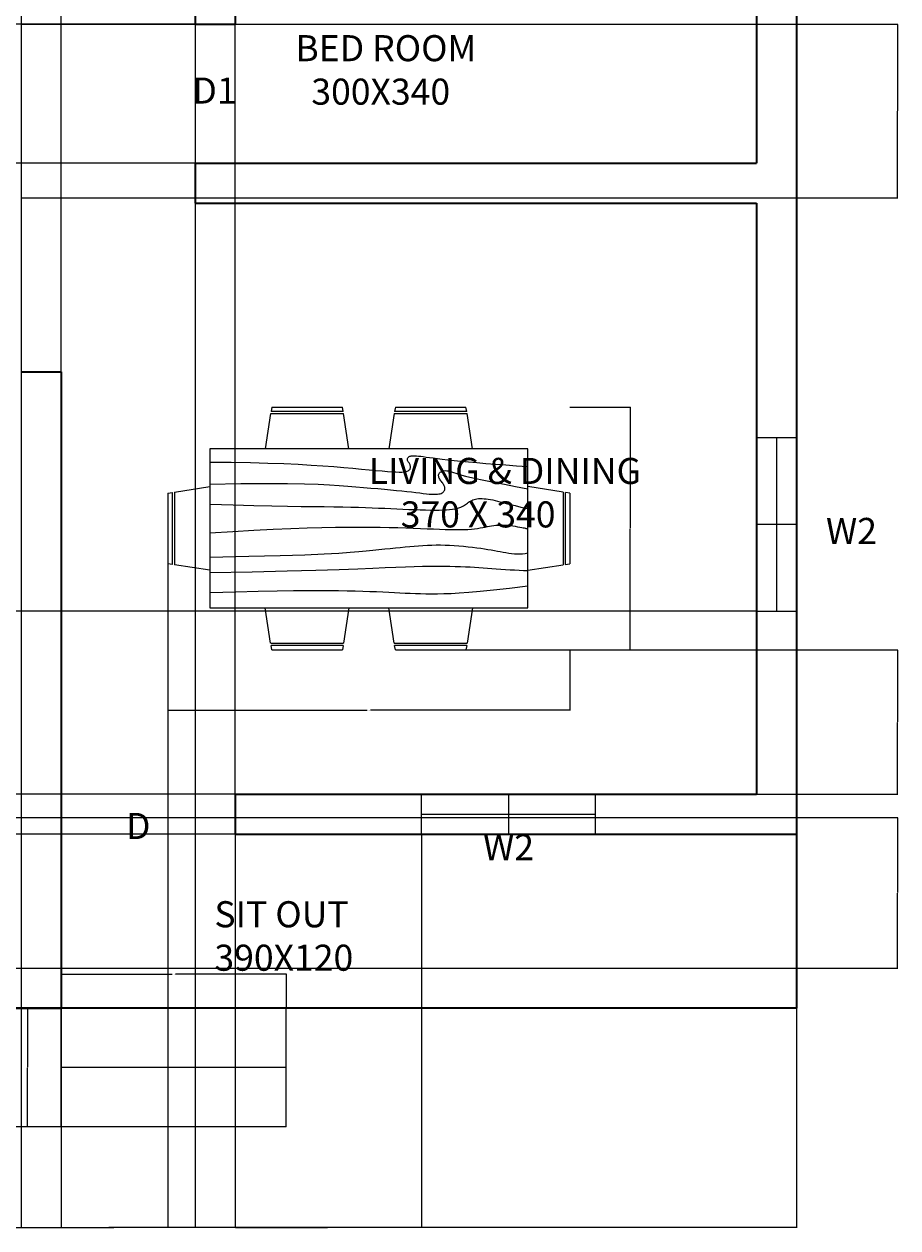
# Model space of a CAD drawing. Units: centimetres. Extents: x 575 to 1481, y 1225 to 2490.
# Tile 2 of 3: x 978 to 1481, y 1225 to 1918. Entities that reach past the tile are written whole.
import ezdxf

# ---------------------------------------------------------------- set-up
doc = ezdxf.new("R2010")
doc.units = ezdxf.units.CM
for name, color, linetype, lineweight in [('A-ANNO-DIMS', 2, 'Continuous', 18), ('A-ANNO-TEXT', 3, 'Continuous', 18), ('A-AREA-IDEN', 7, 'Continuous', 18), ('A-FLOR', 7, 'Continuous', 25), ('A-FLOR-STRS', 7, 'Continuous', 25), ('A-FURN', 8, 'Continuous', 18), ('A-GLAZ', 4, 'Continuous', 18), ('A-WALL', 7, 'Continuous', 35)]:
    doc.layers.add(name, color=color, linetype=linetype, lineweight=lineweight)
doc.styles.get("Standard").update_dxf_attribs({"font": 'arial.ttf'})
doc.dimstyles.get("Standard").update_dxf_attribs({"dimtxt": 0.18, "dimasz": 0.18, "dimexe": 0.18, "dimexo": 0.0625, "dimgap": 0.09, "dimtad": 0, "dimtih": 1, "dimtoh": 1, "dimdec": 4, "dimzin": 0, "dimdsep": 46, "dimtxsty": 'Standard', "dimcen": 0.09, "dimadec": 0, "dimazin": 0, "dimtfac": 1, "dimtdec": 4, "dimtofl": 0, "dimtmove": 0, "dimatfit": 3, "dimfxl": 1, "dimtolj": 1, "dimtzin": 0, "dimarcsym": 0})

# ---------------------------------------------------------------- blocks, each defined once
blk = doc.blocks.new('Dining Set - 36 x 72 in.')
for p, q in [((-22, 27.5), (-22.1562, 26.50042)), ((-22, 27.5), (-6, 27.5)), ((-5.8437, 26.49966), (-6, 27.5)), ((6, 27.5), (5.8438, 26.50042)), ((6, 27.5), (22, 27.5)), ((22.1563, 26.49966), (22, 27.5)), ((-22.2343, 26.00059), (-23.4847, 17.99762)), ((-22.2304, 26), (-5.7608, 26)), ((-5.8416, 26.5), (-22.1534, 26.5)), ((-4.5152, 17.99762), (-5.7655, 25.99926)), ((5.7657, 26.00059), (4.5153, 17.99762)), ((5.7696, 26), (22.2392, 26)), ((22.1584, 26.5), (5.8466, 26.5)), ((23.4848, 17.99762), (22.2345, 25.99926)), ((36, 18), (-36, 18)), ((-36, 18), (-36, -18)), ((36, -18), (36, 18)), ((-44.0006, 8.23428), (-35.9976, 9.48474)), ((-44, 8.23041), (-44, -8.23915)), ((44.0006, 8.23428), (35.9976, 9.48474)), ((44, 8.23041), (44, -8.23915)), ((-45.5, 8), (-44.5004, 8.15617)), ((-45.5, 8), (-45.5, -8)), ((-44.5, -8.15843), (-44.5, 8.15338)), ((44.5, -8.15843), (44.5, 8.15338)), ((45.5, 8), (44.5005, 8.15617)), ((45.5, 8), (45.5, -8)), ((-44.4997, -8.15631), (-45.5, -8)), ((44.4997, -8.15631), (45.5, -8)), ((-35.9976, -9.48476), (-43.9993, -8.2345)), ((35.9976, -9.48476), (43.9993, -8.2345)), ((-36, -18), (36, -18)), ((-22.2343, -26.0006), (-23.4847, -17.99762)), ((-4.5152, -17.99762), (-5.7655, -25.99928)), ((5.7657, -26.0006), (4.5153, -17.99762)), ((23.4848, -17.99762), (22.2345, -25.99928)), ((-22.2304, -26), (-5.7608, -26)), ((-22, -27.5), (-22.1562, -26.50044)), ((-5.8416, -26.5), (-22.1534, -26.5)), ((-5.8437, -26.49967), (-6, -27.5)), ((5.7696, -26), (22.2392, -26)), ((6, -27.5), (5.8438, -26.50044)), ((22.1584, -26.5), (5.8466, -26.5)), ((22.1563, -26.49967), (22, -27.5)), ((-22, -27.5), (-6, -27.5)), ((6, -27.5), (22, -27.5))]:
    blk.add_line(p, q)
for points in [[(-36, 15), (-31.1772, 14.97754), (-26.8079, 14.91406), (-22.8538, 14.81543), (-19.276, 14.6875), (-16.0362, 14.53613), (-13.0957, 14.36718), (-10.4159, 14.18652), (-7.9583, 14), (-5.6904, 13.81315), (-3.6035, 13.63021), (-1.6954, 13.45508), (0.0365, 13.29166), (1.5945, 13.14388), (2.9811, 13.01562), (4.1988, 12.9108), (5.25, 12.83333), (6.1393, 12.78613), (6.8802, 12.76823), (7.4883, 12.77767), (7.9792, 12.8125), (8.3685, 12.87077), (8.6719, 12.95052), (8.9049, 13.0498), (9.0833, 13.16666), (9.2205, 13.29899), (9.3216, 13.44401), (9.3895, 13.59879), (9.4271, 13.76041), (9.4373, 13.92594), (9.4232, 14.09245), (9.3875, 14.257), (9.3333, 14.41666), (9.2638, 14.56917), (9.1836, 14.71484), (9.0975, 14.85465), (9.0104, 14.98958), (8.9272, 15.1206), (8.8529, 15.2487), (8.7922, 15.37483), (8.75, 15.5), (8.7305, 15.62467), (8.7344, 15.74739), (8.7617, 15.86621), (8.8125, 15.97916), (8.8867, 16.08431), (8.9844, 16.17968), (9.1055, 16.26334), (9.25, 16.33333), (9.4189, 16.38802), (9.6172, 16.42708), (9.8506, 16.45052), (10.125, 16.45833), (10.4463, 16.45052), (10.8203, 16.42708), (11.2529, 16.38802), (11.75, 16.33333), (12.3184, 16.26318), (12.9694, 16.17838), (13.7151, 16.07991), (14.5677, 15.96875), (15.5395, 15.84586), (16.6426, 15.71224), (17.8893, 15.56884), (19.2917, 15.41666), (20.859, 15.25667), (22.5879, 15.08984), (24.4721, 14.91715), (26.5052, 14.73958), (28.6809, 14.5581), (30.9929, 14.3737), (33.4347, 14.18733), (36, 14)], [(-36, 10), (-28.9766, 10.14274), (-23.1725, 10.20442), (-18.4241, 10.19775), (-14.5677, 10.13541), (-11.4399, 10.03011), (-8.877, 9.89453), (-6.7154, 9.74137), (-4.7917, 9.58333), (-2.9698, 9.43082), (-1.2246, 9.28515), (0.4415, 9.14534), (2.026, 9.01041), (3.5266, 8.87939), (4.9408, 8.7513), (6.266, 8.62516), (7.5, 8.5), (8.6411, 8.37549), (9.6914, 8.2539), (10.6538, 8.13818), (11.5312, 8.03125), (12.3267, 7.93603), (13.043, 7.85547), (13.6831, 7.79248), (14.25, 7.75), (14.7471, 7.7303), (15.1797, 7.73307), (15.5537, 7.75732), (15.875, 7.80208), (16.1494, 7.86637), (16.3828, 7.94922), (16.5811, 8.04964), (16.75, 8.16666), (16.8944, 8.29915), (17.0143, 8.44531), (17.1089, 8.60319), (17.1771, 8.77083), (17.218, 8.94629), (17.2305, 9.1276), (17.2137, 9.31282), (17.1667, 9.5), (17.0895, 9.6875), (16.987, 9.875), (16.8649, 10.0625), (16.7292, 10.25), (16.5856, 10.4375), (16.4401, 10.625), (16.2985, 10.8125), (16.1667, 11), (16.05, 11.18733), (15.9518, 11.3737), (15.8752, 11.5581), (15.8229, 11.73958), (15.798, 11.91715), (15.8034, 12.08984), (15.842, 12.25667), (15.9167, 12.41666), (16.0295, 12.56836), (16.1784, 12.70833), (16.3605, 12.83268), (16.5729, 12.9375), (16.8127, 13.01888), (17.0768, 13.07291), (17.3625, 13.0957), (17.6667, 13.08333), (17.9894, 13.03312), (18.3418, 12.94726), (18.7382, 12.82918), (19.1927, 12.68229), (19.7195, 12.51001), (20.3327, 12.31575), (21.0465, 12.10294), (21.875, 11.875), (22.8357, 11.63354), (23.959, 11.37304), (25.2786, 11.08618), (26.8282, 10.76562), (28.6414, 10.40405), (30.752, 9.99414), (33.1936, 9.52856), (36, 9)], [(-36, 5.5), (-30.7157, 5.3348), (-26.069, 5.20963), (-21.9946, 5.11767), (-18.4271, 5.05208), (-15.3009, 5.00602), (-12.5508, 4.97265), (-10.1112, 4.94515), (-7.9167, 4.91666), (-5.909, 4.88167), (-4.0586, 4.83984), (-2.3429, 4.79215), (-0.7396, 4.73958), (0.7739, 4.6831), (2.22, 4.6237), (3.6213, 4.56233), (5, 4.5), (6.373, 4.43782), (7.7344, 4.3776), (9.0723, 4.32129), (10.375, 4.27083), (11.6309, 4.22819), (12.8281, 4.19531), (13.9551, 4.17415), (15, 4.16666), (15.954, 4.17448), (16.819, 4.19791), (17.6001, 4.23698), (18.3021, 4.29166), (18.9299, 4.36198), (19.4883, 4.44791), (19.9823, 4.54948), (20.4167, 4.66666), (20.7969, 4.79899), (21.1302, 4.94401), (21.4245, 5.09879), (21.6875, 5.26041), (21.9271, 5.42594), (22.1511, 5.59245), (22.3672, 5.757), (22.5834, 5.91666), (22.8065, 6.06868), (23.0404, 6.21093), (23.2879, 6.34147), (23.5521, 6.45833), (23.8358, 6.55957), (24.142, 6.64323), (24.4735, 6.70735), (24.8334, 6.75), (25.2235, 6.76969), (25.642, 6.76692), (26.0858, 6.74267), (26.5521, 6.69791), (27.0379, 6.63362), (27.5404, 6.55078), (28.0565, 6.45036), (28.5834, 6.33333), (29.1242, 6.19987), (29.7071, 6.04687), (30.3661, 5.87044), (31.1354, 5.66666), (32.0493, 5.43164), (33.142, 5.16146), (34.4475, 4.85221), (36, 4.5)], [(-36, -1), (-30.7915, -0.6591), (-26.0195, -0.38216), (-21.6519, -0.16284), (-17.6563, 0.00521), (-14.0005, 0.12833), (-10.6523, 0.21289), (-7.5796, 0.26522), (-4.75, 0.29166), (-2.134, 0.29793), (0.2878, 0.28711), (2.5317, 0.26163), (4.6146, 0.22396), (6.5529, 0.17651), (8.3633, 0.12174), (10.0623, 0.06209), (11.6667, 0), (13.1899, -0.06201), (14.6341, -0.1211), (15.9982, -0.17432), (17.2813, -0.21875), (18.4823, -0.25147), (19.6003, -0.26953), (20.6343, -0.27002), (21.5834, -0.25), (22.4481, -0.20768), (23.2357, -0.14584), (23.9549, -0.06836), (24.6146, 0.02083), (25.2235, 0.11784), (25.7904, 0.21875), (26.3241, 0.31966), (26.8334, 0.41666), (27.3265, 0.50618), (27.8099, 0.58593), (28.2894, 0.65397), (28.7709, 0.70833), (29.2601, 0.74707), (29.763, 0.76823), (30.2855, 0.76985), (30.8334, 0.75), (31.4088, 0.70784), (31.9994, 0.64713), (32.589, 0.57275), (33.1615, 0.48958), (33.7008, 0.4025), (34.1908, 0.3164), (34.6153, 0.23616), (34.9584, 0.16666), (35.2099, 0.11165), (35.3848, 0.07031), (35.504, 0.04069), (35.5886, 0.02083), (35.6594, 0.00879), (35.7377, 0.0026), (35.8442, 0.00032), (36, 0)], [(-36, -6.5), (-27.1843, -6.31267), (-20.084, -6.1263), (-14.469, -5.9419), (-10.1094, -5.76042), (-6.7752, -5.58285), (-4.2363, -5.41016), (-2.2629, -5.24333), (-0.625, -5.08334), (0.8708, -4.93099), (2.2715, -4.78646), (3.5872, -4.64974), (4.8281, -4.52084), (6.0046, -4.39974), (7.127, -4.28646), (8.2053, -4.18099), (9.25, -4.08334), (10.2705, -3.99382), (11.2734, -3.91407), (12.2647, -3.84603), (13.25, -3.79167), (14.2354, -3.75293), (15.2266, -3.73177), (16.2295, -3.73015), (17.25, -3.75), (18.2912, -3.79248), (19.3451, -3.85547), (20.4009, -3.93604), (21.4479, -4.03125), (22.4754, -4.13819), (23.4727, -4.25391), (24.4289, -4.37549), (25.3334, -4.5), (26.1785, -4.62492), (26.9694, -4.74935), (27.7145, -4.87281), (28.4219, -4.99479), (29.1, -5.11483), (29.7572, -5.23242), (30.4016, -5.34709), (31.0417, -5.45834), (31.6837, -5.56437), (32.3262, -5.65821), (32.9658, -5.73153), (33.599, -5.77604), (34.2224, -5.78345), (34.8327, -5.74545), (35.4264, -5.65373), (36, -5.5)], [(-36, -10), (-26.4022, -9.81299), (-18.4675, -9.62891), (-11.9839, -9.45069), (-6.7396, -9.28125), (-2.5226, -9.12354), (0.8789, -8.98047), (3.6769, -8.85498), (6.0833, -8.75), (8.2767, -8.66765), (10.3021, -8.60677), (12.1712, -8.56543), (13.8958, -8.54167), (15.4876, -8.53353), (16.9583, -8.53907), (18.3197, -8.55632), (19.5834, -8.58334), (20.7616, -8.61841), (21.8685, -8.66081), (22.9188, -8.71004), (23.9271, -8.76563), (24.9081, -8.82707), (25.8763, -8.89388), (26.8465, -8.96558), (27.8334, -9.04167), (28.8474, -9.12118), (29.8828, -9.20117), (30.93, -9.27824), (31.9792, -9.34896), (33.0205, -9.40991), (34.0443, -9.45768), (35.0407, -9.48885), (36, -9.5)], [(-36, -14.5), (-30.0881, -14.33513), (-25.0332, -14.21224), (-20.7312, -14.12647), (-17.0781, -14.07292), (-13.97, -14.04671), (-11.3027, -14.04297), (-8.9724, -14.05681), (-6.875, -14.08334), (-4.9224, -14.11833), (-3.0905, -14.16016), (-1.3709, -14.20785), (0.2448, -14.26042), (1.7647, -14.3169), (3.1973, -14.3763), (4.5507, -14.43767), (5.8333, -14.5), (7.0554, -14.5621), (8.235, -14.62175), (9.3922, -14.67652), (10.5469, -14.72396), (11.7192, -14.76164), (12.929, -14.78711), (14.1965, -14.79794), (15.5417, -14.79167), (16.9933, -14.76424), (18.6152, -14.70508), (20.4804, -14.60197), (22.6615, -14.44271), (25.2312, -14.21509), (28.2624, -13.9069), (31.8277, -13.50594), (36, -13)]]:
    blk.add_lwpolyline(points)
blk = doc.blocks.new('WIN-W2-100CM')
for p, q in [((0, 0), (0, 23)), ((50, 23), (50, 0)), ((100, 0), (100, 23)), ((0, 11.5), (100, 11.5))]:
    blk.add_line(p, q)
blk = doc.blocks.new('ENTRY-STEPS')
for p, q in [((0, 0), (0, 68.38)), ((129.45, 68.38), (0, 68.38)), ((129.45, 0), (129.45, 68.38)), ((129.45, 34.19), (0, 34.19)), ((129.45, 0), (0, 0))]:
    blk.add_line(p, q)
blk = doc.blocks.new('*D16')
at = {"layer": 'A-ANNO-DIMS', "color": 0, "lineweight": -2, "transparency": 16777216}
for p, q in [((999.46, 1351.63), (999.46, 1371.16)), ((999.64, 1370.98), (1063.14, 1370.98)), ((1128.73, 1370.98), (1065.23, 1370.98)), ((1128.91, 1351.63), (1128.91, 1371.16))]:
    blk.add_line(p, q, dxfattribs=at)
at = {"layer": 'A-ANNO-DIMS', "color": 0, "transparency": 16777216}
for points in [[(999.64, 1371.01), (999.64, 1370.95), (999.46, 1370.98)], [(1128.73, 1371.01), (1128.73, 1370.95), (1128.91, 1370.98)]]:
    blk.add_solid(points, dxfattribs=at)
at = {"layer": 'Defpoints', "color": 0, "transparency": 16777216}
for p in [(1128.91, 1370.98), (999.46, 1351.57), (1128.91, 1351.57)]:
    blk.add_point(p, dxfattribs=at)
at = {"layer": 'A-ANNO-DIMS', "color": 0, "transparency": 16777216, "insert": (1064.18, 1370.98), "char_height": 0.18, "attachment_point": 5}
blk.add_mtext('\\A1;STEPS 129 TYP.', dxfattribs=at)
blk = doc.blocks.new('*D17')
at = {"layer": 'A-ANNO-DIMS', "color": 0, "lineweight": -2, "transparency": 16777216}
for p, q in [((999.39, 1351.57), (979.86, 1351.57)), ((980.04, 1351.39), (980.04, 1317.56)), ((980.04, 1283.37), (980.04, 1317.19)), ((999.39, 1283.19), (979.86, 1283.19))]:
    blk.add_line(p, q, dxfattribs=at)
at = {"layer": 'A-ANNO-DIMS', "color": 0, "transparency": 16777216}
for points in [[(980.01, 1351.39), (980.07, 1351.39), (980.04, 1351.57)], [(980.01, 1283.37), (980.07, 1283.37), (980.04, 1283.19)]]:
    blk.add_solid(points, dxfattribs=at)
at = {"layer": 'Defpoints', "color": 0, "transparency": 16777216}
for p in [(980.04, 1351.57), (999.46, 1351.57), (999.46, 1283.19)]:
    blk.add_point(p, dxfattribs=at)
at = {"layer": 'A-ANNO-DIMS', "color": 0, "transparency": 16777216, "insert": (980.04, 1317.38), "char_height": 0.18, "attachment_point": 5}
blk.add_mtext('\\A1;68 TYP.', dxfattribs=at)
blk = doc.blocks.new('*D22')
at = {"layer": 'A-ANNO-DIMS', "color": 0, "lineweight": -2, "transparency": 16777216}
for p, q in [((1060.8, 1557.52), (1060.8, 1522.73)), ((1291.94, 1557.52), (1291.94, 1522.73)), ((1060.98, 1522.91), (1175.35, 1522.91)), ((1291.76, 1522.91), (1177.39, 1522.91))]:
    blk.add_line(p, q, dxfattribs=at)
at = {"layer": 'A-ANNO-DIMS', "color": 0, "transparency": 16777216}
for points in [[(1060.98, 1522.94), (1060.98, 1522.88), (1060.8, 1522.91)], [(1291.76, 1522.94), (1291.76, 1522.88), (1291.94, 1522.91)]]:
    blk.add_solid(points, dxfattribs=at)
at = {"layer": 'Defpoints', "color": 0, "transparency": 16777216}
for p in [(1060.8, 1557.58), (1291.94, 1557.58), (1291.94, 1522.91)]:
    blk.add_point(p, dxfattribs=at)
at = {"layer": 'A-ANNO-DIMS', "color": 0, "transparency": 16777216, "insert": (1176.37, 1522.91), "char_height": 0.18, "attachment_point": 5}
blk.add_mtext('\\A1;DINING SET 231', dxfattribs=at)
blk = doc.blocks.new('*D23')
at = {"layer": 'A-ANNO-DIMS', "color": 0, "lineweight": -2, "transparency": 16777216}
for p, q in [((1292, 1697.28), (1326.79, 1697.28)), ((1326.61, 1697.1), (1326.61, 1627.61)), ((1326.61, 1557.76), (1326.61, 1627.25)), ((1292, 1557.58), (1326.79, 1557.58))]:
    blk.add_line(p, q, dxfattribs=at)
at = {"layer": 'A-ANNO-DIMS', "color": 0, "transparency": 16777216}
for points in [[(1326.58, 1697.1), (1326.64, 1697.1), (1326.61, 1697.28)], [(1326.58, 1557.76), (1326.64, 1557.76), (1326.61, 1557.58)]]:
    blk.add_solid(points, dxfattribs=at)
at = {"layer": 'Defpoints', "color": 0, "transparency": 16777216}
for p in [(1291.94, 1697.28), (1326.61, 1697.28), (1291.94, 1557.58)]:
    blk.add_point(p, dxfattribs=at)
at = {"layer": 'A-ANNO-DIMS', "color": 0, "transparency": 16777216, "insert": (1326.61, 1627.43), "char_height": 0.18, "attachment_point": 5}
blk.add_mtext('\\A1;140', dxfattribs=at)
blk = doc.blocks.new('*D28')
at = {"layer": 'A-ANNO-DIMS', "color": 0, "lineweight": -2, "transparency": 16777216}
for p, q in [((633.46, 1351.5), (633.46, 1225.06)), ((1422.46, 1351.5), (1422.46, 1225.06)), ((633.64, 1225.24), (1027.67, 1225.24)), ((1422.28, 1225.24), (1028.25, 1225.24))]:
    blk.add_line(p, q, dxfattribs=at)
at = {"layer": 'A-ANNO-DIMS', "color": 0, "transparency": 16777216}
for points in [[(633.64, 1225.27), (633.64, 1225.21), (633.46, 1225.24)], [(1422.28, 1225.27), (1422.28, 1225.21), (1422.46, 1225.24)]]:
    blk.add_solid(points, dxfattribs=at)
at = {"layer": 'Defpoints', "color": 0, "transparency": 16777216}
for p in [(633.46, 1351.57), (1422.46, 1351.57), (1422.46, 1225.24)]:
    blk.add_point(p, dxfattribs=at)
at = {"layer": 'A-ANNO-DIMS', "color": 0, "transparency": 16777216, "insert": (1027.96, 1225.24), "char_height": 0.18, "attachment_point": 5}
blk.add_mtext('\\A1;789', dxfattribs=at)
blk = doc.blocks.new('*D29')
at = {"layer": 'A-ANNO-DIMS', "color": 0, "lineweight": -2, "transparency": 16777216}
for p, q in [((959.64, 2431.95), (575.33, 2431.95)), ((575.51, 2431.77), (575.51, 1857.75)), ((575.51, 1283.37), (575.51, 1857.38)), ((999.39, 1283.19), (575.33, 1283.19))]:
    blk.add_line(p, q, dxfattribs=at)
at = {"layer": 'A-ANNO-DIMS', "color": 0, "transparency": 16777216}
for points in [[(575.48, 2431.77), (575.54, 2431.77), (575.51, 2431.95)], [(575.48, 1283.37), (575.54, 1283.37), (575.51, 1283.19)]]:
    blk.add_solid(points, dxfattribs=at)
at = {"layer": 'Defpoints', "color": 0, "transparency": 16777216}
for p in [(575.51, 2431.95), (959.71, 2431.95), (999.46, 1283.19)]:
    blk.add_point(p, dxfattribs=at)
at = {"layer": 'A-ANNO-DIMS', "color": 0, "transparency": 16777216, "insert": (575.51, 1857.57), "char_height": 0.18, "attachment_point": 5}
blk.add_mtext('\\A1;1148.8', dxfattribs=at)
blk = doc.blocks.new('*D31')
at = {"layer": 'A-ANNO-DIMS', "color": 0, "lineweight": -2, "transparency": 16777216}
for p, q in [((1099.46, 1451.5), (1099.46, 1225.06)), ((1206.74, 1451.5), (1206.74, 1225.06)), ((1099.64, 1225.24), (1152.64, 1225.24)), ((1206.56, 1225.24), (1153.55, 1225.24))]:
    blk.add_line(p, q, dxfattribs=at)
at = {"layer": 'A-ANNO-DIMS', "color": 0, "transparency": 16777216}
for points in [[(1099.64, 1225.27), (1099.64, 1225.21), (1099.46, 1225.24)], [(1206.56, 1225.27), (1206.56, 1225.21), (1206.74, 1225.24)]]:
    blk.add_solid(points, dxfattribs=at)
at = {"layer": 'Defpoints', "color": 0, "transparency": 16777216}
for p in [(1099.46, 1451.57), (1206.74, 1451.57), (1206.74, 1225.24)]:
    blk.add_point(p, dxfattribs=at)
at = {"layer": 'A-ANNO-DIMS', "color": 0, "transparency": 16777216, "insert": (1153.1, 1225.24), "char_height": 0.18, "attachment_point": 5}
blk.add_mtext('\\A1;107.28', dxfattribs=at)
blk = doc.blocks.new('*D32')
at = {"layer": 'A-ANNO-DIMS', "color": 0, "lineweight": -2, "transparency": 16777216}
for p, q in [((656.52, 1461.2), (1480.59, 1461.2)), ((1480.41, 1461.02), (1480.41, 1418.07)), ((1480.41, 1374.75), (1480.41, 1417.7)), ((656.52, 1374.57), (1480.59, 1374.57))]:
    blk.add_line(p, q, dxfattribs=at)
at = {"layer": 'A-ANNO-DIMS', "color": 0, "transparency": 16777216}
for points in [[(1480.38, 1461.02), (1480.44, 1461.02), (1480.41, 1461.2)], [(1480.38, 1374.75), (1480.44, 1374.75), (1480.41, 1374.57)]]:
    blk.add_solid(points, dxfattribs=at)
at = {"layer": 'Defpoints', "color": 0, "transparency": 16777216}
for p in [(656.46, 1461.2), (1480.41, 1461.2), (656.46, 1374.57)]:
    blk.add_point(p, dxfattribs=at)
at = {"layer": 'A-ANNO-DIMS', "color": 0, "transparency": 16777216, "insert": (1480.41, 1417.88), "char_height": 0.18, "attachment_point": 5}
blk.add_mtext('\\A1;86.63', dxfattribs=at)
blk = doc.blocks.new('*D37')
at = {"layer": 'A-ANNO-DIMS', "color": 0, "lineweight": -2, "transparency": 16777216}
for p, q in [((1076.46, 2363.5), (1076.46, 1225.06)), ((976.46, 2340.5), (976.46, 1225.06)), ((976.64, 1225.24), (1026.18, 1225.24)), ((1076.28, 1225.24), (1026.74, 1225.24))]:
    blk.add_line(p, q, dxfattribs=at)
at = {"layer": 'A-ANNO-DIMS', "color": 0, "transparency": 16777216}
for points in [[(976.64, 1225.27), (976.64, 1225.21), (976.46, 1225.24)], [(1076.28, 1225.27), (1076.28, 1225.21), (1076.46, 1225.24)]]:
    blk.add_solid(points, dxfattribs=at)
at = {"layer": 'Defpoints', "color": 0, "transparency": 16777216}
for p in [(1076.46, 2363.57), (976.46, 2340.57), (1076.46, 1225.24)]:
    blk.add_point(p, dxfattribs=at)
at = {"layer": 'A-ANNO-DIMS', "color": 0, "transparency": 16777216, "insert": (1026.46, 1225.24), "char_height": 0.18, "attachment_point": 5}
blk.add_mtext('\\A1;100', dxfattribs=at)
blk = doc.blocks.new('*D39')
at = {"layer": 'A-ANNO-DIMS', "color": 0, "lineweight": -2, "transparency": 16777216}
for p, q in [((1399.39, 1579.79), (575.33, 1579.79)), ((575.51, 1579.61), (575.51, 1527.36)), ((575.51, 1474.75), (575.51, 1527)), ((1399.39, 1474.57), (575.33, 1474.57))]:
    blk.add_line(p, q, dxfattribs=at)
at = {"layer": 'A-ANNO-DIMS', "color": 0, "transparency": 16777216}
for points in [[(575.48, 1579.61), (575.54, 1579.61), (575.51, 1579.79)], [(575.48, 1474.75), (575.54, 1474.75), (575.51, 1474.57)]]:
    blk.add_solid(points, dxfattribs=at)
at = {"layer": 'Defpoints', "color": 0, "transparency": 16777216}
for p in [(575.51, 1579.79), (1399.46, 1579.79), (1399.46, 1474.57)]:
    blk.add_point(p, dxfattribs=at)
at = {"layer": 'A-ANNO-DIMS', "color": 0, "transparency": 16777216, "insert": (575.51, 1527.18), "char_height": 0.18, "attachment_point": 5}
blk.add_mtext('\\A1;105.22', dxfattribs=at)
blk = doc.blocks.new('*D40')
at = {"layer": 'A-ANNO-DIMS', "color": 0, "lineweight": -2, "transparency": 16777216}
for p, q in [((1399.39, 1925.38), (575.33, 1925.38)), ((575.51, 1925.2), (575.51, 1881.66)), ((575.51, 1837.75), (575.51, 1881.29)), ((1399.39, 1837.57), (575.33, 1837.57))]:
    blk.add_line(p, q, dxfattribs=at)
at = {"layer": 'A-ANNO-DIMS', "color": 0, "transparency": 16777216}
for points in [[(575.48, 1925.2), (575.54, 1925.2), (575.51, 1925.38)], [(575.48, 1837.75), (575.54, 1837.75), (575.51, 1837.57)]]:
    blk.add_solid(points, dxfattribs=at)
at = {"layer": 'Defpoints', "color": 0, "transparency": 16777216}
for p in [(575.51, 1925.38), (1399.46, 1925.38), (1399.46, 1837.57)]:
    blk.add_point(p, dxfattribs=at)
at = {"layer": 'A-ANNO-DIMS', "color": 0, "transparency": 16777216, "insert": (575.51, 1881.47), "char_height": 0.18, "attachment_point": 5}
blk.add_mtext('\\A1;87.82', dxfattribs=at)
blk = doc.blocks.new('*D42')
at = {"layer": 'A-ANNO-DIMS', "color": 0, "lineweight": -2, "transparency": 16777216}
for p, q in [((976.52, 1917.57), (1480.59, 1917.57)), ((1480.41, 1917.39), (1480.41, 1867.75)), ((1480.41, 1817.75), (1480.41, 1867.38)), ((976.52, 1817.57), (1480.59, 1817.57))]:
    blk.add_line(p, q, dxfattribs=at)
at = {"layer": 'A-ANNO-DIMS', "color": 0, "transparency": 16777216}
for points in [[(1480.38, 1917.39), (1480.44, 1917.39), (1480.41, 1917.57)], [(1480.38, 1817.75), (1480.44, 1817.75), (1480.41, 1817.57)]]:
    blk.add_solid(points, dxfattribs=at)
at = {"layer": 'Defpoints', "color": 0, "transparency": 16777216}
for p in [(976.46, 1917.57), (1480.41, 1917.57), (976.46, 1817.57)]:
    blk.add_point(p, dxfattribs=at)
at = {"layer": 'A-ANNO-DIMS', "color": 0, "transparency": 16777216, "insert": (1480.41, 1867.57), "char_height": 0.18, "attachment_point": 5}
blk.add_mtext('\\A1;100', dxfattribs=at)
blk = doc.blocks.new('*D46')
at = {"layer": 'A-ANNO-DIMS', "color": 0, "lineweight": -2, "transparency": 16777216}
for p, q in [((1076.39, 1917.57), (575.33, 1917.57)), ((575.51, 1917.39), (575.51, 1877.75)), ((575.51, 1837.75), (575.51, 1877.38)), ((1076.39, 1837.57), (575.33, 1837.57))]:
    blk.add_line(p, q, dxfattribs=at)
at = {"layer": 'A-ANNO-DIMS', "color": 0, "transparency": 16777216}
for points in [[(575.48, 1917.39), (575.54, 1917.39), (575.51, 1917.57)], [(575.48, 1837.75), (575.54, 1837.75), (575.51, 1837.57)]]:
    blk.add_solid(points, dxfattribs=at)
at = {"layer": 'Defpoints', "color": 0, "transparency": 16777216}
for p in [(575.51, 1917.57), (1076.46, 1917.57), (1076.46, 1837.57)]:
    blk.add_point(p, dxfattribs=at)
at = {"layer": 'A-ANNO-DIMS', "color": 0, "transparency": 16777216, "insert": (575.51, 1877.57), "char_height": 0.18, "attachment_point": 5}
blk.add_mtext('\\A1;80', dxfattribs=at)
blk = doc.blocks.new('*D48')
at = {"layer": 'A-ANNO-DIMS', "color": 0, "lineweight": -2, "transparency": 16777216}
for p, q in [((999.46, 1351.63), (999.46, 2490.08)), ((999.64, 2489.9), (1049.18, 2489.9)), ((1099.28, 2489.9), (1049.74, 2489.9)), ((1099.46, 1451.63), (1099.46, 2490.08))]:
    blk.add_line(p, q, dxfattribs=at)
at = {"layer": 'A-ANNO-DIMS', "color": 0, "transparency": 16777216}
for points in [[(999.64, 2489.93), (999.64, 2489.87), (999.46, 2489.9)], [(1099.28, 2489.93), (1099.28, 2489.87), (1099.46, 2489.9)]]:
    blk.add_solid(points, dxfattribs=at)
at = {"layer": 'Defpoints', "color": 0, "transparency": 16777216}
for p in [(1099.46, 2489.9), (1099.46, 1451.57), (999.46, 1351.57)]:
    blk.add_point(p, dxfattribs=at)
at = {"layer": 'A-ANNO-DIMS', "color": 0, "transparency": 16777216, "insert": (1049.46, 2489.9), "char_height": 0.18, "attachment_point": 5}
blk.add_mtext('\\A1;100', dxfattribs=at)
blk = doc.blocks.new('*D55')
at = {"layer": 'A-ANNO-DIMS', "color": 0, "lineweight": -2, "transparency": 16777216}
for p, q in [((999.46, 1717.5), (999.46, 1225.06)), ((1060.8, 1607.05), (1060.8, 1225.06)), ((999.64, 1225.24), (1029.73, 1225.24)), ((1060.62, 1225.24), (1030.52, 1225.24))]:
    blk.add_line(p, q, dxfattribs=at)
at = {"layer": 'A-ANNO-DIMS', "color": 0, "transparency": 16777216}
for points in [[(999.64, 1225.27), (999.64, 1225.21), (999.46, 1225.24)], [(1060.62, 1225.27), (1060.62, 1225.21), (1060.8, 1225.24)]]:
    blk.add_solid(points, dxfattribs=at)
at = {"layer": 'Defpoints', "color": 0, "transparency": 16777216}
for p in [(999.46, 1717.57), (1060.8, 1607.11), (1060.8, 1225.24)]:
    blk.add_point(p, dxfattribs=at)
at = {"layer": 'A-ANNO-DIMS', "color": 0, "transparency": 16777216, "insert": (1030.13, 1225.24), "char_height": 0.18, "attachment_point": 5}
blk.add_mtext('\\A1;61.34', dxfattribs=at)
blk = doc.blocks.new('*D56')
at = {"layer": 'A-ANNO-DIMS', "color": 0, "lineweight": -2, "transparency": 16777216}
for p, q in [((1232.31, 1557.58), (1480.59, 1557.58)), ((1480.41, 1557.4), (1480.41, 1516.25)), ((1480.41, 1474.75), (1480.41, 1515.89)), ((1399.52, 1474.57), (1480.59, 1474.57))]:
    blk.add_line(p, q, dxfattribs=at)
at = {"layer": 'A-ANNO-DIMS', "color": 0, "transparency": 16777216}
for points in [[(1480.38, 1557.4), (1480.44, 1557.4), (1480.41, 1557.58)], [(1480.38, 1474.75), (1480.44, 1474.75), (1480.41, 1474.57)]]:
    blk.add_solid(points, dxfattribs=at)
at = {"layer": 'Defpoints', "color": 0, "transparency": 16777216}
for p in [(1232.25, 1557.58), (1480.41, 1557.58), (1399.46, 1474.57)]:
    blk.add_point(p, dxfattribs=at)
at = {"layer": 'A-ANNO-DIMS', "color": 0, "transparency": 16777216, "insert": (1480.41, 1516.07), "char_height": 0.18, "attachment_point": 5}
blk.add_mtext('\\A1;83.01', dxfattribs=at)
blk = doc.blocks.new('*D57')
at = {"layer": 'A-ANNO-DIMS', "color": 0, "lineweight": -2, "transparency": 16777216}
for p, q in [((1422.39, 1451.57), (575.33, 1451.57)), ((575.51, 1451.39), (575.51, 1401.75)), ((575.51, 1351.75), (575.51, 1401.38)), ((1422.39, 1351.57), (575.33, 1351.57))]:
    blk.add_line(p, q, dxfattribs=at)
at = {"layer": 'A-ANNO-DIMS', "color": 0, "transparency": 16777216}
for points in [[(575.48, 1451.39), (575.54, 1451.39), (575.51, 1451.57)], [(575.48, 1351.75), (575.54, 1351.75), (575.51, 1351.57)]]:
    blk.add_solid(points, dxfattribs=at)
at = {"layer": 'Defpoints', "color": 0, "transparency": 16777216}
for p in [(575.51, 1451.57), (1422.46, 1451.57), (1422.46, 1351.57)]:
    blk.add_point(p, dxfattribs=at)
at = {"layer": 'A-ANNO-DIMS', "color": 0, "transparency": 16777216, "insert": (575.51, 1401.57), "char_height": 0.18, "attachment_point": 5}
blk.add_mtext('\\A1;100', dxfattribs=at)

msp = doc.modelspace()

# ---------------------------------------------------------------- linework, layer by layer
at = {"layer": 'A-FLOR'}
msp.add_line((999.457, 1351.566), (1422.457, 1351.566), dxfattribs=at)
at = {"layer": 'A-GLAZ'}
for p, q in [((1399.457, 1679.7906), (1399.457, 1579.7906)), ((1422.457, 1579.7906), (1422.457, 1679.7906))]:
    msp.add_line(p, q, dxfattribs=at)
at = {"layer": 'A-WALL'}
for p, q in [((1076.457, 2363.566), (1076.457, 1917.566)), ((1422.457, 2363.566), (1422.457, 1351.566)), ((1399.457, 2340.566), (1399.457, 1837.566)), ((1099.457, 2177.566), (1099.457, 1917.566)), ((1076.457, 1917.566), (1099.457, 1917.566)), ((1076.457, 1837.566), (1399.457, 1837.566)), ((1076.457, 1837.566), (1076.457, 1814.566)), ((1076.457, 1814.566), (1399.457, 1814.566)), ((1399.457, 1814.566), (1399.457, 1474.566)), ((976.457, 1717.566), (999.457, 1717.566)), ((999.457, 1717.566), (999.457, 1351.566)), ((1099.457, 1474.566), (1399.457, 1474.566)), ((1099.457, 1474.566), (1099.457, 1451.566)), ((1099.457, 1451.566), (1422.457, 1451.566)), ((633.457, 1351.566), (999.457, 1351.566))]:
    msp.add_line(p, q, dxfattribs=at)

# ---------------------------------------------------------------- block references
at = {"layer": 'A-FLOR-STRS'}
msp.add_blockref('ENTRY-STEPS', (999.4565, 1283.1864), dxfattribs=at)
at = {"layer": 'A-FURN', "xscale": 2.54, "yscale": 2.54, "zscale": 2.54}
msp.add_blockref('Dining Set - 36 x 72 in.', (1176.3676, 1627.4299), dxfattribs=at)
at = {"layer": 'A-GLAZ', "rotation": 269.9999999999999}
msp.add_blockref('WIN-W2-100CM', (1399.4569, 1679.7901), dxfattribs=at)
at = {"layer": 'A-GLAZ'}
msp.add_blockref('WIN-W2-100CM', (1206.739, 1451.566), dxfattribs=at)

# ---------------------------------------------------------------- texts
at = {"layer": 'A-ANNO-TEXT', "char_height": 15, "attachment_point": 1}
for s, insert in [('D1', (1074.889, 1886.824)), ('W2', (1439.3315, 1633.4884)), ('D', (1036.6686, 1463.7707)), ('W2', (1242.0708, 1451.566))]:
    msp.add_mtext_dynamic_manual_height_columns(s, width=230.89075, gutter_width=12.5, heights=[0], dxfattribs=dict(at, insert=insert))
at = {"layer": 'A-AREA-IDEN', "char_height": 15, "attachment_point": 1}
for s, heights, insert in [('BED ROOM\\P  300X340', [68.7606], (1134.1082, 1911.2008)), ('LIVING & DINING\\P    370 X 340', [0], (1176.3676, 1668.0132)), ('SIT OUT \\P390X120', [0], (1087.5366, 1412.9951))]:
    msp.add_mtext_dynamic_manual_height_columns(s, width=230.89075, gutter_width=12.5, heights=heights, dxfattribs=dict(at, insert=insert))

# ---------------------------------------------------------------- dimensions: what is measured, and where the dimension line sits
at = {"layer": 'A-ANNO-DIMS'}
for base, p1, p2, override, picture, middle in [((1099.457, 2489.8956), (999.457, 1351.566), (1099.457, 1451.566), {"dimdec": 0, "dimlfac": 1, "dimrnd": 0, "dimzin": 0, "dimdsep": 46, "dimlunit": 2}, '*D48', (1049.457, 2489.8956)), ((1076.457, 1225.2364), (976.457, 2340.566), (1076.457, 2363.566), {"dimdec": 0, "dimlfac": 1, "dimrnd": 0, "dimzin": 0, "dimdsep": 46, "dimlunit": 2}, '*D37', (1026.457, 1225.2364)), ((1060.7976, 1225.2364), (999.457, 1717.566), (1060.7976, 1607.1099), {"dimdec": 2, "dimlfac": 1, "dimrnd": 0, "dimzin": 0, "dimdsep": 46, "dimlunit": 2}, '*D55', (1030.1273, 1225.2364)), ((1206.7385, 1225.2364), (1099.457, 1451.566), (1206.7385, 1451.566), {"dimdec": 2, "dimlfac": 1, "dimrnd": 0, "dimzin": 0, "dimdsep": 46, "dimlunit": 2}, '*D31', (1153.0978, 1225.2364)), ((1422.457, 1225.2364), (633.457, 1351.566), (1422.457, 1351.566), {"dimdec": 0, "dimlfac": 1, "dimrnd": 0, "dimzin": 0, "dimdsep": 46, "dimlunit": 2}, '*D28', (1027.957, 1225.2364))]:
    dim = msp.add_linear_dim(base=base, p1=p1, p2=p2, dimstyle='Standard', override=override, dxfattribs=at)
    dim.commit()
    dim.dimension.update_dxf_attribs({"geometry": picture, "text_midpoint": middle})
for base, p1, p2, override, picture, middle in [((575.507, 2431.9456), (999.457, 1283.1864), (959.7054, 2431.9456), {"dimdec": 1, "dimlfac": 1, "dimrnd": 0, "dimzin": 0, "dimdsep": 46, "dimlunit": 2}, '*D29', (575.507, 1857.566)), ((575.507, 1925.3838), (1399.457, 1837.566), (1399.457, 1925.3838), {"dimdec": 2, "dimlfac": 1, "dimrnd": 0, "dimzin": 0, "dimdsep": 46, "dimlunit": 2}, '*D40', (575.507, 1881.4749)), ((575.507, 1917.566), (1076.457, 1837.566), (1076.457, 1917.566), {"dimdec": 0, "dimlfac": 1, "dimrnd": 0, "dimzin": 0, "dimdsep": 46, "dimlunit": 2}, '*D46', (575.507, 1877.566)), ((1480.407, 1917.566), (976.457, 1817.566), (976.457, 1917.566), {"dimdec": 0, "dimlfac": 1, "dimrnd": 0, "dimzin": 0, "dimdsep": 46, "dimlunit": 2}, '*D42', (1480.407, 1867.566)), ((1326.6086, 1697.2799), (1291.9376, 1557.5799), (1291.9376, 1697.2799), {"dimdec": 0, "dimlfac": 1, "dimrnd": 0, "dimzin": 0, "dimdsep": 46, "dimlunit": 2}, '*D23', (1326.6086, 1627.4299)), ((575.507, 1579.7906), (1399.457, 1474.566), (1399.457, 1579.7906), {"dimdec": 2, "dimlfac": 1, "dimrnd": 0, "dimzin": 0, "dimdsep": 46, "dimlunit": 2}, '*D39', (575.507, 1527.1783)), ((1480.407, 1557.5799), (1399.457, 1474.566), (1232.2476, 1557.5799), {"dimdec": 2, "dimlfac": 1, "dimrnd": 0, "dimzin": 0, "dimdsep": 46, "dimlunit": 2}, '*D56', (1480.407, 1516.073)), ((1480.407, 1461.2007), (656.457, 1374.566), (656.457, 1461.2007), {"dimdec": 2, "dimlfac": 1, "dimrnd": 0, "dimzin": 0, "dimdsep": 46, "dimlunit": 2}, '*D32', (1480.407, 1417.8834)), ((575.507, 1451.566), (1422.457, 1351.566), (1422.457, 1451.566), {"dimdec": 0, "dimlfac": 1, "dimrnd": 0, "dimzin": 0, "dimdsep": 46, "dimlunit": 2}, '*D57', (575.507, 1401.566))]:
    dim = msp.add_linear_dim(base=base, p1=p1, p2=p2, angle=90, dimstyle='Standard', override=override, dxfattribs=at)
    dim.commit()
    dim.dimension.update_dxf_attribs({"geometry": picture, "text_midpoint": middle})
for base, p1, p2, text, picture, middle in [((1291.9376, 1522.9089), (1060.7976, 1557.5799), (1291.9376, 1557.5799), 'DINING SET <>', '*D22', (1176.3676, 1522.9089)), ((1128.9053, 1370.9833), (999.457, 1351.566), (1128.9053, 1351.566), 'STEPS <> TYP.', '*D16', (1064.1811, 1370.9833))]:
    dim = msp.add_linear_dim(base=base, p1=p1, p2=p2, text=text, dimstyle='Standard', override={"dimdec": 0, "dimlfac": 1, "dimrnd": 0, "dimzin": 0, "dimdsep": 46, "dimlunit": 2}, dxfattribs=at)
    dim.commit()
    dim.dimension.update_dxf_attribs({"geometry": picture, "text_midpoint": middle})
dim = msp.add_linear_dim(base=(980.0397, 1351.566), p1=(999.457, 1283.1864), p2=(999.457, 1351.566), angle=90, text='<> TYP.', dimstyle='Standard', override={"dimdec": 0, "dimlfac": 1, "dimrnd": 0, "dimzin": 0, "dimdsep": 46, "dimlunit": 2}, dxfattribs=at)
dim.commit()
dim.dimension.update_dxf_attribs({"geometry": '*D17', "text_midpoint": (980.0397, 1317.3762)})

doc.saveas('drawing.dxf')
